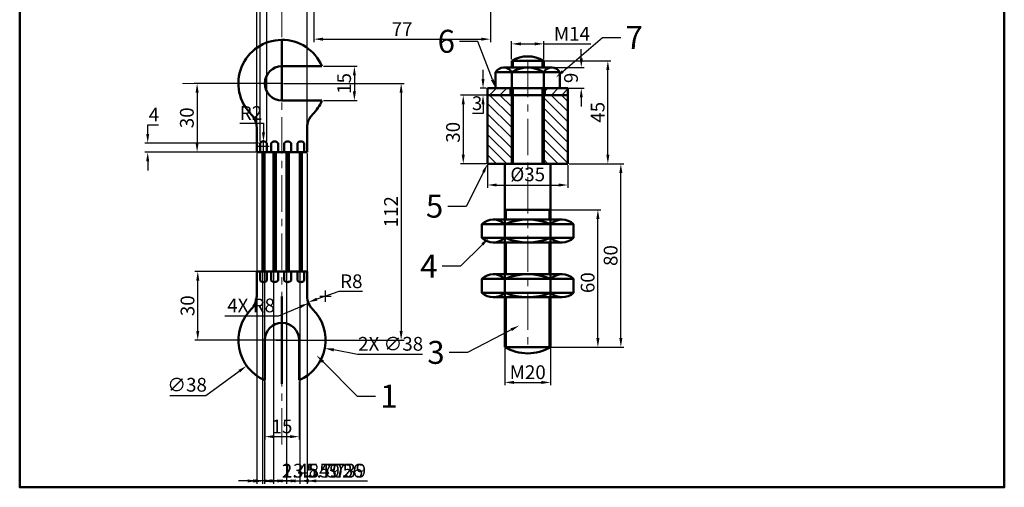
# Model space of a CAD drawing. Units: millimetres. Extents: x 297 to 727, y 87 to 537.
# Tile 1 of 2: x 297 to 727, y 87 to 291. Entities that reach past the tile are written whole.
import ezdxf
from ezdxf import colors
from ezdxf.entities.mleader import LeaderData, LeaderLine
from ezdxf.math import Vec2, Vec3

# ---------------------------------------------------------------- set-up
doc = ezdxf.new("R2010")
doc.units = ezdxf.units.MM
doc.header["$LTSCALE"] = 0.5
doc.linetypes.add('CENTER', pattern=[50.8, 31.75, -6.35, 6.35, -6.35])
for name, color, linetype, lineweight in [('M-CNTR', 1, 'CENTER', 18), ('M-DIMS', 2, 'Continuous', 25), ('M-HATC', 8, 'Continuous', 18), ('M-OUTL', 7, 'Continuous', 50), ('M-TEXT', 3, 'Continuous', 25), ('M-TTLB', 7, 'Continuous', 50)]:
    doc.layers.add(name, color=color, linetype=linetype, lineweight=lineweight)
doc.styles.get("Standard").update_dxf_attribs({"font": 'arial.ttf'})
doc.dimstyles.new('ISO-25', dxfattribs={"dimtxt": 6, "dimasz": 4, "dimexe": 1.25, "dimexo": 0.625, "dimtad": 1, "dimtoh": 1, "dimtxsty": 'Standard', "dimcen": 2.5, "dimadec": 0, "dimazin": 0, "dimtfac": 1, "dimtofl": 0, "dimtmove": 0, "dimatfit": 3, "dimfxl": 1, "dimarcsym": 0})

# ---------------------------------------------------------------- blocks, each defined once
blk = doc.blocks.new('*D1')
at = {"layer": 'Defpoints', "color": 0, "transparency": 16777216}
for p in [(525.99, 280.54), (511.99, 273.2), (525.99, 273.2)]:
    blk.add_point(p, dxfattribs=at)
at = {"layer": 'M-DIMS', "color": 0, "lineweight": -2, "transparency": 16777216}
for p, q in [((511.99, 273.83), (511.99, 281.79)), ((515.99, 280.54), (521.99, 280.54)), ((525.99, 273.83), (525.99, 281.79)), ((525.99, 280.54), (546.52, 280.54))]:
    blk.add_line(p, q, dxfattribs=at)
at = {"layer": 'M-DIMS', "color": 0, "transparency": 16777216}
for points in [[(515.99, 281.21), (515.99, 279.88), (511.99, 280.54)], [(521.99, 281.21), (521.99, 279.88), (525.99, 280.54)]]:
    blk.add_solid(points, dxfattribs=at)
at = {"layer": 'M-DIMS', "color": 0, "transparency": 16777216, "insert": (538.26, 284.18), "char_height": 6, "attachment_point": 5}
blk.add_mtext('M14', dxfattribs=at)
blk = doc.blocks.new('*D2')
at = {"layer": 'Defpoints', "color": 0, "transparency": 16777216}
for p in [(508.38, 270.2), (542.34, 270.2), (504.99, 261.2)]:
    blk.add_point(p, dxfattribs=at)
at = {"layer": 'M-DIMS', "color": 0, "lineweight": -2, "transparency": 16777216}
for p, q in [((542.34, 274.2), (542.34, 278.2)), ((509.01, 270.2), (543.59, 270.2)), ((505.62, 261.2), (543.59, 261.2)), ((542.34, 257.2), (542.34, 253.2))]:
    blk.add_line(p, q, dxfattribs=at)
at = {"layer": 'M-DIMS', "color": 0, "transparency": 16777216}
for points in [[(541.68, 274.2), (543.01, 274.2), (542.34, 270.2)], [(541.68, 257.2), (543.01, 257.2), (542.34, 261.2)]]:
    blk.add_solid(points, dxfattribs=at)
at = {"layer": 'M-DIMS', "color": 0, "transparency": 16777216, "insert": (538.66, 265.7), "char_height": 6, "attachment_point": 5, "rotation": 90}
blk.add_mtext('9', dxfattribs=at)
blk = doc.blocks.new('*D3')
at = {"layer": 'Defpoints', "color": 0, "transparency": 16777216}
for p in [(499.5, 258.2), (501.49, 261.2), (501.49, 258.2)]:
    blk.add_point(p, dxfattribs=at)
at = {"layer": 'M-DIMS', "color": 0, "lineweight": -2, "transparency": 16777216}
for p, q in [((499.5, 265.2), (499.5, 269.2)), ((500.87, 261.2), (498.25, 261.2)), ((500.87, 258.2), (498.25, 258.2)), ((499.5, 254.2), (499.5, 250.2)), ((499.5, 250.2), (494.95, 250.2))]:
    blk.add_line(p, q, dxfattribs=at)
at = {"layer": 'M-DIMS', "color": 0, "transparency": 16777216}
for points in [[(498.83, 265.2), (500.17, 265.2), (499.5, 261.2)], [(498.83, 254.2), (500.17, 254.2), (499.5, 258.2)]]:
    blk.add_solid(points, dxfattribs=at)
at = {"layer": 'M-DIMS', "color": 0, "transparency": 16777216, "insert": (496.91, 253.89), "char_height": 6, "attachment_point": 5}
blk.add_mtext('3', dxfattribs=at)
blk = doc.blocks.new('*D4')
at = {"layer": 'Defpoints', "color": 0, "transparency": 16777216}
for p in [(501.49, 258.2), (490.87, 228.2), (501.49, 228.2)]:
    blk.add_point(p, dxfattribs=at)
at = {"layer": 'M-DIMS', "color": 0, "lineweight": -2, "transparency": 16777216}
for p, q in [((500.87, 258.2), (489.62, 258.2)), ((490.87, 254.2), (490.87, 232.2)), ((500.87, 228.2), (489.62, 228.2))]:
    blk.add_line(p, q, dxfattribs=at)
at = {"layer": 'M-DIMS', "color": 0, "transparency": 16777216}
for points in [[(490.21, 254.2), (491.54, 254.2), (490.87, 258.2)], [(490.21, 232.2), (491.54, 232.2), (490.87, 228.2)]]:
    blk.add_solid(points, dxfattribs=at)
at = {"layer": 'M-DIMS', "color": 0, "transparency": 16777216, "insert": (487.18, 241.96), "char_height": 6, "attachment_point": 5, "rotation": 90}
blk.add_mtext('30', dxfattribs=at)
blk = doc.blocks.new('*D5')
at = {"layer": 'Defpoints', "color": 0, "transparency": 16777216}
for p in [(518.99, 273.2), (553.94, 273.2), (536.49, 228.2)]:
    blk.add_point(p, dxfattribs=at)
at = {"layer": 'M-DIMS', "color": 0, "lineweight": -2, "transparency": 16777216}
for p, q in [((519.62, 273.2), (555.19, 273.2)), ((553.94, 232.2), (553.94, 269.2)), ((537.12, 228.2), (555.19, 228.2))]:
    blk.add_line(p, q, dxfattribs=at)
at = {"layer": 'M-DIMS', "color": 0, "transparency": 16777216}
for points in [[(553.27, 269.2), (554.6, 269.2), (553.94, 273.2)], [(553.27, 232.2), (554.6, 232.2), (553.94, 228.2)]]:
    blk.add_solid(points, dxfattribs=at)
at = {"layer": 'M-DIMS', "color": 0, "transparency": 16777216, "insert": (550.26, 250.7), "char_height": 6, "attachment_point": 5, "rotation": 90}
blk.add_mtext('45', dxfattribs=at)
blk = doc.blocks.new('*D6')
at = {"layer": 'Defpoints', "color": 0, "transparency": 16777216}
for p in [(501.49, 228.2), (536.49, 228.2), (536.49, 218.97)]:
    blk.add_point(p, dxfattribs=at)
at = {"layer": 'M-DIMS', "color": 0, "lineweight": -2, "transparency": 16777216}
for p, q in [((501.49, 227.58), (501.49, 217.72)), ((536.49, 227.58), (536.49, 217.72)), ((505.49, 218.97), (532.49, 218.97))]:
    blk.add_line(p, q, dxfattribs=at)
at = {"layer": 'M-DIMS', "color": 0, "transparency": 16777216}
for points in [[(505.49, 219.63), (505.49, 218.3), (501.49, 218.97)], [(532.49, 219.63), (532.49, 218.3), (536.49, 218.97)]]:
    blk.add_solid(points, dxfattribs=at)
at = {"layer": 'M-DIMS', "color": 0, "transparency": 16777216, "insert": (518.99, 222.82), "char_height": 6, "attachment_point": 5}
blk.add_mtext('%%C35', dxfattribs=at)
blk = doc.blocks.new('*D7')
at = {"layer": 'Defpoints', "color": 0, "transparency": 16777216}
for p in [(518.99, 208.2), (549.59, 208.2), (518.99, 148.2)]:
    blk.add_point(p, dxfattribs=at)
at = {"layer": 'M-DIMS', "color": 0, "lineweight": -2, "transparency": 16777216}
for p, q in [((519.62, 208.2), (550.84, 208.2)), ((549.59, 152.2), (549.59, 204.2)), ((519.62, 148.2), (550.84, 148.2))]:
    blk.add_line(p, q, dxfattribs=at)
at = {"layer": 'M-DIMS', "color": 0, "transparency": 16777216}
for points in [[(548.92, 204.2), (550.26, 204.2), (549.59, 208.2)], [(548.92, 152.2), (550.26, 152.2), (549.59, 148.2)]]:
    blk.add_solid(points, dxfattribs=at)
at = {"layer": 'M-DIMS', "color": 0, "transparency": 16777216, "insert": (545.9, 176.36), "char_height": 6, "attachment_point": 5, "rotation": 90}
blk.add_mtext('60', dxfattribs=at)
blk = doc.blocks.new('*D8')
at = {"layer": 'Defpoints', "color": 0, "transparency": 16777216}
for p in [(536.49, 228.2), (559.61, 228.2), (518.99, 148.2)]:
    blk.add_point(p, dxfattribs=at)
at = {"layer": 'M-DIMS', "color": 0, "lineweight": -2, "transparency": 16777216}
for p, q in [((537.12, 228.2), (560.86, 228.2)), ((559.61, 152.2), (559.61, 224.2)), ((519.62, 148.2), (560.86, 148.2))]:
    blk.add_line(p, q, dxfattribs=at)
at = {"layer": 'M-DIMS', "color": 0, "transparency": 16777216}
for points in [[(558.94, 224.2), (560.28, 224.2), (559.61, 228.2)], [(558.94, 152.2), (560.28, 152.2), (559.61, 148.2)]]:
    blk.add_solid(points, dxfattribs=at)
at = {"layer": 'M-DIMS', "color": 0, "transparency": 16777216, "insert": (555.92, 188.2), "char_height": 6, "attachment_point": 5, "rotation": 90}
blk.add_mtext('80', dxfattribs=at)
blk = doc.blocks.new('*D9')
at = {"layer": 'Defpoints', "color": 0, "transparency": 16777216}
for p in [(508.99, 148.2), (528.99, 148.2), (528.99, 132.83)]:
    blk.add_point(p, dxfattribs=at)
at = {"layer": 'M-DIMS', "color": 0, "lineweight": -2, "transparency": 16777216}
for p, q in [((508.99, 147.58), (508.99, 131.58)), ((528.99, 147.58), (528.99, 131.58)), ((512.99, 132.83), (524.99, 132.83))]:
    blk.add_line(p, q, dxfattribs=at)
at = {"layer": 'M-DIMS', "color": 0, "transparency": 16777216}
for points in [[(512.99, 133.5), (512.99, 132.17), (508.99, 132.83)], [(524.99, 133.5), (524.99, 132.17), (528.99, 132.83)]]:
    blk.add_solid(points, dxfattribs=at)
at = {"layer": 'M-DIMS', "color": 0, "transparency": 16777216, "insert": (518.99, 136.52), "char_height": 6, "attachment_point": 5}
blk.add_mtext('M20', dxfattribs=at)
blk = doc.blocks.new('*D10')
at = {"layer": 'Defpoints', "color": 0, "transparency": 16777216}
for p in [(429.27, 270.79), (429.27, 255.79), (443.4, 255.79)]:
    blk.add_point(p, dxfattribs=at)
at = {"layer": 'M-DIMS', "color": 0, "lineweight": -2, "transparency": 16777216}
for p, q in [((429.9, 270.79), (444.65, 270.79)), ((443.4, 266.79), (443.4, 259.79)), ((429.9, 255.79), (444.65, 255.79))]:
    blk.add_line(p, q, dxfattribs=at)
at = {"layer": 'M-DIMS', "color": 0, "transparency": 16777216}
for points in [[(442.74, 266.79), (444.07, 266.79), (443.4, 270.79)], [(442.74, 259.79), (444.07, 259.79), (443.4, 255.79)]]:
    blk.add_solid(points, dxfattribs=at)
at = {"layer": 'M-DIMS', "color": 0, "transparency": 16777216, "insert": (439.71, 263.29), "char_height": 6, "attachment_point": 5, "rotation": 90}
blk.add_mtext('15', dxfattribs=at)
blk = doc.blocks.new('*D11')
at = {"layer": 'Defpoints', "color": 0, "transparency": 16777216}
for p in [(411.82, 263.29), (374.81, 233.29), (411.82, 233.29)]:
    blk.add_point(p, dxfattribs=at)
at = {"layer": 'M-DIMS', "color": 0, "lineweight": -2, "transparency": 16777216}
for p, q in [((411.19, 263.29), (373.56, 263.29)), ((374.81, 259.29), (374.81, 237.29)), ((411.19, 233.29), (373.56, 233.29))]:
    blk.add_line(p, q, dxfattribs=at)
at = {"layer": 'M-DIMS', "color": 0, "transparency": 16777216}
for points in [[(374.14, 259.29), (375.48, 259.29), (374.81, 263.29)], [(374.14, 237.29), (375.48, 237.29), (374.81, 233.29)]]:
    blk.add_solid(points, dxfattribs=at)
at = {"layer": 'M-DIMS', "color": 0, "transparency": 16777216, "insert": (371.12, 248.29), "char_height": 6, "attachment_point": 5, "rotation": 90}
blk.add_mtext('30', dxfattribs=at)
blk = doc.blocks.new('*D12')
at = {"layer": 'Defpoints', "color": 0, "transparency": 16777216}
for p in [(375.1, 181.29), (411.82, 181.29), (411.82, 151.29)]:
    blk.add_point(p, dxfattribs=at)
at = {"layer": 'M-DIMS', "color": 0, "lineweight": -2, "transparency": 16777216}
for p, q in [((411.19, 181.29), (373.85, 181.29)), ((375.1, 155.29), (375.1, 177.29)), ((411.19, 151.29), (373.85, 151.29))]:
    blk.add_line(p, q, dxfattribs=at)
at = {"layer": 'M-DIMS', "color": 0, "transparency": 16777216}
for points in [[(374.44, 177.29), (375.77, 177.29), (375.1, 181.29)], [(374.44, 155.29), (375.77, 155.29), (375.1, 151.29)]]:
    blk.add_solid(points, dxfattribs=at)
at = {"layer": 'M-DIMS', "color": 0, "transparency": 16777216, "insert": (371.41, 166.29), "char_height": 6, "attachment_point": 5, "rotation": 90}
blk.add_mtext('30', dxfattribs=at)
blk = doc.blocks.new('*D13')
at = {"layer": 'Defpoints', "color": 0, "transparency": 16777216}
for p in [(404.32, 133.83), (419.32, 133.83), (419.32, 109.19)]:
    blk.add_point(p, dxfattribs=at)
at = {"layer": 'M-DIMS', "color": 0, "lineweight": -2, "transparency": 16777216}
for p, q in [((404.32, 133.21), (404.32, 107.94)), ((419.32, 133.21), (419.32, 107.94)), ((408.32, 109.19), (415.32, 109.19))]:
    blk.add_line(p, q, dxfattribs=at)
at = {"layer": 'M-DIMS', "color": 0, "transparency": 16777216}
for points in [[(408.32, 109.85), (408.32, 108.52), (404.32, 109.19)], [(415.32, 109.85), (415.32, 108.52), (419.32, 109.19)]]:
    blk.add_solid(points, dxfattribs=at)
at = {"layer": 'M-DIMS', "color": 0, "transparency": 16777216, "insert": (411.82, 112.88), "char_height": 6, "attachment_point": 5}
blk.add_mtext('15', dxfattribs=at)
blk = doc.blocks.new('*D14')
at = {"layer": 'Defpoints', "color": 0, "transparency": 16777216}
for p in [(427.19, 162.46), (396.45, 140.12)]:
    blk.add_point(p, dxfattribs=at)
at = {"layer": 'M-DIMS', "color": 0, "lineweight": -2, "transparency": 16777216}
for p, q in [((409.32, 151.29), (414.32, 151.29)), ((411.82, 148.79), (411.82, 153.79)), ((378.65, 127.19), (393.21, 137.77)), ((362.89, 127.19), (378.65, 127.19))]:
    blk.add_line(p, q, dxfattribs=at)
at = {"layer": 'M-DIMS', "color": 0, "transparency": 16777216}
blk.add_solid([(392.82, 138.31), (393.6, 137.23), (396.45, 140.12)], dxfattribs=at)
at = {"layer": 'M-DIMS', "color": 0, "transparency": 16777216, "insert": (370.45, 131.04), "char_height": 6, "attachment_point": 5}
blk.add_mtext('∅38', dxfattribs=at)
blk = doc.blocks.new('*D15')
at = {"layer": 'Defpoints', "color": 0, "transparency": 16777216}
for p in [(423.27, 167.83), (430.82, 170.48)]:
    blk.add_point(p, dxfattribs=at)
at = {"layer": 'M-DIMS', "color": 0, "lineweight": -2, "transparency": 16777216}
for p, q in [((436.6, 172.5), (427.04, 169.15)), ((446.91, 172.5), (436.6, 172.5))]:
    blk.add_line(p, q, dxfattribs=at)
at = {"layer": 'M-DIMS', "color": 0, "transparency": 16777216}
blk.add_solid([(426.82, 169.78), (427.26, 168.52), (423.27, 167.83)], dxfattribs=at)
at = {"layer": 'M-DIMS', "color": 0, "transparency": 16777216, "insert": (442.07, 176.19), "char_height": 6, "attachment_point": 5}
blk.add_mtext('R8', dxfattribs=at)
blk = doc.blocks.new('*D16')
at = {"layer": 'Defpoints', "color": 0, "ltscale": 0.5, "transparency": 16777216}
for p in [(411.82, 263.29), (411.82, 151.29), (463.8, 151.29)]:
    blk.add_point(p, dxfattribs=at)
at = {"layer": 'M-DIMS', "color": 0, "lineweight": -2, "ltscale": 0.5, "transparency": 16777216}
for p, q in [((412.44, 263.29), (465.05, 263.29)), ((463.8, 259.29), (463.8, 155.29)), ((412.44, 151.29), (465.05, 151.29))]:
    blk.add_line(p, q, dxfattribs=at)
at = {"layer": 'M-DIMS', "color": 0, "ltscale": 0.5, "transparency": 16777216}
for points in [[(463.13, 259.29), (464.46, 259.29), (463.8, 263.29)], [(463.13, 155.29), (464.46, 155.29), (463.8, 151.29)]]:
    blk.add_solid(points, dxfattribs=at)
at = {"layer": 'M-DIMS', "color": 0, "ltscale": 0.5, "transparency": 16777216, "insert": (460.16, 207.29), "char_height": 6, "attachment_point": 5, "rotation": 90}
blk.add_mtext('112', dxfattribs=at)
blk = doc.blocks.new('NUT-HEX-M20')
for p, q in [((30, 2), (30, 10)), ((0, 2), (0, 8)), ((0, 8), (40, 8)), ((10, 2), (10, 8)), ((40, 8), (40, 2)), ((40, 2), (0, 2))]:
    blk.add_line(p, q)
for centre, radius, start, end in [((5, 2.75), 7.25, 46.3972, 133.6028), ((20, -16), 26, 67.3801, 112.6199), ((35, 2.75), 7.25, 46.3972, 133.6028), ((5, 7.25), 7.25, 226.3972, 313.6028), ((20, 26), 26, 247.3801, 292.6199), ((35, 7.25), 7.25, 226.3972, 313.6028)]:
    blk.add_arc(centre, radius, start, end)
blk = doc.blocks.new('WIRE-STRAND-END')
for p, q in [((0, 4.68), (0, 0.68)), ((3, 0.68), (3, 4.68))]:
    blk.add_line(p, q)
blk.add_arc((1.5, 2), 2, 221.4096, 318.5904)
blk = doc.blocks.new('BOLT-END-DOME')
for p, q in [((0, 3), (0, 0)), ((0, 3), (14, 3)), ((14, 3), (14, 0))]:
    blk.add_line(p, q)
blk.add_arc((7, -9.12), 14, 60, 120)
blk = doc.blocks.new('*D23')
at = {"layer": 'Defpoints', "color": 0, "ltscale": 0.5, "transparency": 16777216}
for p in [(425.71, 301.75), (502.71, 303.24), (502.71, 282.6)]:
    blk.add_point(p, dxfattribs=at)
at = {"layer": 'M-DIMS', "color": 0, "lineweight": -2, "ltscale": 0.5, "transparency": 16777216}
for p, q in [((425.71, 301.12), (425.71, 281.35)), ((502.71, 302.61), (502.71, 281.35)), ((429.71, 282.6), (498.71, 282.6))]:
    blk.add_line(p, q, dxfattribs=at)
at = {"layer": 'M-DIMS', "color": 0, "ltscale": 0.5, "transparency": 16777216}
for points in [[(429.71, 283.27), (429.71, 281.93), (425.71, 282.6)], [(498.71, 283.27), (498.71, 281.93), (502.71, 282.6)]]:
    blk.add_solid(points, dxfattribs=at)
at = {"layer": 'M-DIMS', "color": 0, "ltscale": 0.5, "transparency": 16777216, "insert": (464.21, 286.22), "char_height": 6, "attachment_point": 5}
blk.add_mtext('77', dxfattribs=at)
blk = doc.blocks.new('*D28')
at = {"layer": 'Defpoints', "color": 0, "ltscale": 0.5, "transparency": 16777216}
for p in [(422.82, 314.56), (400.82, 244.11), (422.82, 244.11)]:
    blk.add_point(p, dxfattribs=at)
at = {"layer": 'M-DIMS', "color": 0, "lineweight": -2, "ltscale": 0.5, "transparency": 16777216}
for p, q in [((400.82, 244.73), (400.82, 315.81)), ((404.82, 314.56), (418.82, 314.56)), ((422.82, 244.73), (422.82, 315.81))]:
    blk.add_line(p, q, dxfattribs=at)
at = {"layer": 'M-DIMS', "color": 0, "ltscale": 0.5, "transparency": 16777216}
for points in [[(404.82, 315.23), (404.82, 313.89), (400.82, 314.56)], [(418.82, 315.23), (418.82, 313.89), (422.82, 314.56)]]:
    blk.add_solid(points, dxfattribs=at)
at = {"layer": 'M-DIMS', "color": 0, "ltscale": 0.5, "transparency": 16777216, "insert": (411.82, 318.2), "char_height": 6, "attachment_point": 5}
blk.add_mtext('22', dxfattribs=at)
blk = doc.blocks.new('*D29')
at = {"layer": 'Defpoints', "color": 0, "ltscale": 0.5, "transparency": 16777216}
for p in [(400.82, 233.29), (403.26, 233.29), (403.26, 89.87)]:
    blk.add_point(p, dxfattribs=at)
at = {"layer": 'M-DIMS', "color": 0, "lineweight": -2, "ltscale": 0.5, "transparency": 16777216}
for p, q in [((400.82, 232.67), (400.82, 88.62)), ((403.26, 232.67), (403.26, 88.62)), ((396.82, 89.87), (392.82, 89.87)), ((407.26, 89.87), (428.24, 89.87))]:
    blk.add_line(p, q, dxfattribs=at)
at = {"layer": 'M-DIMS', "color": 0, "ltscale": 0.5, "transparency": 16777216}
for points in [[(396.82, 90.54), (396.82, 89.2), (400.82, 89.87)], [(407.26, 90.54), (407.26, 89.2), (403.26, 89.87)]]:
    blk.add_solid(points, dxfattribs=at)
at = {"layer": 'M-DIMS', "color": 0, "ltscale": 0.5, "transparency": 16777216, "insert": (419.75, 93.56), "char_height": 6, "attachment_point": 5}
blk.add_mtext('2.45', dxfattribs=at)
blk = doc.blocks.new('*D30')
at = {"layer": 'Defpoints', "color": 0, "ltscale": 0.5, "transparency": 16777216}
for p in [(403.26, 233.29), (404.26, 233.29), (404.26, 89.87)]:
    blk.add_point(p, dxfattribs=at)
at = {"layer": 'M-DIMS', "color": 0, "lineweight": -2, "ltscale": 0.5, "transparency": 16777216}
for p, q in [((403.26, 232.67), (403.26, 88.62)), ((404.26, 232.67), (404.26, 88.62)), ((399.26, 89.87), (395.26, 89.87)), ((408.26, 89.87), (415.72, 89.87))]:
    blk.add_line(p, q, dxfattribs=at)
at = {"layer": 'M-DIMS', "color": 0, "ltscale": 0.5, "transparency": 16777216}
for points in [[(399.26, 90.54), (399.26, 89.2), (403.26, 89.87)], [(408.26, 90.54), (408.26, 89.2), (404.26, 89.87)]]:
    blk.add_solid(points, dxfattribs=at)
at = {"layer": 'M-DIMS', "color": 0, "ltscale": 0.5, "transparency": 16777216, "insert": (413.99, 93.51), "char_height": 6, "attachment_point": 5}
blk.add_mtext('1', dxfattribs=at)
blk = doc.blocks.new('*D31')
at = {"layer": 'Defpoints', "color": 0, "ltscale": 0.5, "transparency": 16777216}
for p in [(404.26, 233.29), (408.11, 233.29), (408.11, 89.87)]:
    blk.add_point(p, dxfattribs=at)
at = {"layer": 'M-DIMS', "color": 0, "lineweight": -2, "ltscale": 0.5, "transparency": 16777216}
for p, q in [((404.26, 232.67), (404.26, 88.62)), ((408.11, 232.67), (408.11, 88.62)), ((400.26, 89.87), (396.26, 89.87)), ((412.11, 89.87), (437.62, 89.87))]:
    blk.add_line(p, q, dxfattribs=at)
at = {"layer": 'M-DIMS', "color": 0, "ltscale": 0.5, "transparency": 16777216}
for points in [[(400.26, 90.54), (400.26, 89.2), (404.26, 89.87)], [(412.11, 90.54), (412.11, 89.2), (408.11, 89.87)]]:
    blk.add_solid(points, dxfattribs=at)
at = {"layer": 'M-DIMS', "color": 0, "ltscale": 0.5, "transparency": 16777216, "insert": (426.86, 93.56), "char_height": 6, "attachment_point": 5}
blk.add_mtext('3.849', dxfattribs=at)
blk = doc.blocks.new('*D32')
at = {"layer": 'Defpoints', "color": 0, "ltscale": 0.5, "transparency": 16777216}
for p in [(408.11, 233.29), (413.82, 233.29), (413.82, 89.87)]:
    blk.add_point(p, dxfattribs=at)
at = {"layer": 'M-DIMS', "color": 0, "lineweight": -2, "ltscale": 0.5, "transparency": 16777216}
for p, q in [((408.11, 232.67), (408.11, 88.62)), ((413.82, 232.67), (413.82, 88.62)), ((404.11, 89.87), (400.11, 89.87)), ((417.82, 89.87), (443.36, 89.87))]:
    blk.add_line(p, q, dxfattribs=at)
at = {"layer": 'M-DIMS', "color": 0, "ltscale": 0.5, "transparency": 16777216}
for points in [[(404.11, 90.54), (404.11, 89.2), (408.11, 89.87)], [(417.82, 90.54), (417.82, 89.2), (413.82, 89.87)]]:
    blk.add_solid(points, dxfattribs=at)
at = {"layer": 'M-DIMS', "color": 0, "ltscale": 0.5, "transparency": 16777216, "insert": (432.59, 93.56), "char_height": 6, "attachment_point": 5}
blk.add_mtext('5.705', dxfattribs=at)
blk = doc.blocks.new('*D33')
at = {"layer": 'Defpoints', "color": 0, "ltscale": 0.5, "transparency": 16777216}
for p in [(413.82, 233.29), (419.55, 233.29), (419.55, 89.87)]:
    blk.add_point(p, dxfattribs=at)
at = {"layer": 'M-DIMS', "color": 0, "lineweight": -2, "ltscale": 0.5, "transparency": 16777216}
for p, q in [((413.82, 232.67), (413.82, 88.62)), ((419.55, 232.67), (419.55, 88.62)), ((409.82, 89.87), (405.82, 89.87)), ((423.55, 89.87), (449.06, 89.87))]:
    blk.add_line(p, q, dxfattribs=at)
at = {"layer": 'M-DIMS', "color": 0, "ltscale": 0.5, "transparency": 16777216}
for points in [[(409.82, 90.54), (409.82, 89.2), (413.82, 89.87)], [(423.55, 90.54), (423.55, 89.2), (419.55, 89.87)]]:
    blk.add_solid(points, dxfattribs=at)
at = {"layer": 'M-DIMS', "color": 0, "ltscale": 0.5, "transparency": 16777216, "insert": (438.31, 93.56), "char_height": 6, "attachment_point": 5}
blk.add_mtext('5.739', dxfattribs=at)
blk = doc.blocks.new('*D34')
at = {"layer": 'Defpoints', "color": 0, "ltscale": 0.5, "transparency": 16777216}
for p in [(419.55, 233.29), (422.82, 233.29), (422.82, 89.87)]:
    blk.add_point(p, dxfattribs=at)
at = {"layer": 'M-DIMS', "color": 0, "lineweight": -2, "ltscale": 0.5, "transparency": 16777216}
for p, q in [((419.55, 232.67), (419.55, 88.62)), ((422.82, 232.67), (422.82, 88.62)), ((415.55, 89.87), (411.55, 89.87)), ((426.82, 89.87), (447.64, 89.87))]:
    blk.add_line(p, q, dxfattribs=at)
at = {"layer": 'M-DIMS', "color": 0, "ltscale": 0.5, "transparency": 16777216}
for points in [[(415.55, 90.54), (415.55, 89.2), (419.55, 89.87)], [(426.82, 90.54), (426.82, 89.2), (422.82, 89.87)]]:
    blk.add_solid(points, dxfattribs=at)
at = {"layer": 'M-DIMS', "color": 0, "ltscale": 0.5, "transparency": 16777216, "insert": (439.23, 93.56), "char_height": 6, "attachment_point": 5}
blk.add_mtext('3.26', dxfattribs=at)
blk = doc.blocks.new('*D35')
at = {"layer": 'Defpoints', "color": 0, "ltscale": 0.5, "transparency": 16777216}
for p in [(405.26, 314.56), (402.26, 237.29), (405.26, 237.29)]:
    blk.add_point(p, dxfattribs=at)
at = {"layer": 'M-DIMS', "color": 0, "lineweight": -2, "ltscale": 0.5, "transparency": 16777216}
for p, q in [((398.26, 314.56), (394.26, 314.56)), ((402.26, 237.92), (402.26, 315.81)), ((405.26, 237.92), (405.26, 315.81)), ((409.26, 314.56), (418.44, 314.56))]:
    blk.add_line(p, q, dxfattribs=at)
at = {"layer": 'M-DIMS', "color": 0, "ltscale": 0.5, "transparency": 16777216}
for points in [[(398.26, 315.23), (398.26, 313.89), (402.26, 314.56)], [(409.26, 315.23), (409.26, 313.89), (405.26, 314.56)]]:
    blk.add_solid(points, dxfattribs=at)
at = {"layer": 'M-DIMS', "color": 0, "ltscale": 0.5, "transparency": 16777216, "insert": (415.85, 318.25), "char_height": 6, "attachment_point": 5}
blk.add_mtext('3', dxfattribs=at)
blk = doc.blocks.new('*D36')
at = {"layer": 'Defpoints', "color": 0, "ltscale": 0.5, "transparency": 16777216}
for p in [(353.28, 237.29), (402.26, 237.29), (402.26, 233.29)]:
    blk.add_point(p, dxfattribs=at)
at = {"layer": 'M-DIMS', "color": 0, "lineweight": -2, "ltscale": 0.5, "transparency": 16777216}
for p, q in [((353.28, 241.29), (353.28, 245.29)), ((353.28, 245.29), (358.05, 245.29)), ((401.64, 237.29), (352.03, 237.29)), ((401.64, 233.29), (352.03, 233.29)), ((353.28, 229.29), (353.28, 225.29))]:
    blk.add_line(p, q, dxfattribs=at)
at = {"layer": 'M-DIMS', "color": 0, "ltscale": 0.5, "transparency": 16777216}
for points in [[(352.61, 241.29), (353.94, 241.29), (353.28, 237.29)], [(352.61, 229.29), (353.94, 229.29), (353.28, 233.29)]]:
    blk.add_solid(points, dxfattribs=at)
at = {"layer": 'M-DIMS', "color": 0, "ltscale": 0.5, "transparency": 16777216, "insert": (355.98, 248.92), "char_height": 6, "attachment_point": 5}
blk.add_mtext('4', dxfattribs=at)
blk = doc.blocks.new('*D43')
at = {"layer": 'Defpoints', "color": 0, "ltscale": 0.5, "transparency": 16777216}
for p in [(393.15, 154.83), (430.48, 147.75)]:
    blk.add_point(p, dxfattribs=at)
at = {"layer": 'M-DIMS', "color": 0, "lineweight": -2, "ltscale": 0.5, "transparency": 16777216}
for p, q in [((409.32, 151.29), (414.32, 151.29)), ((411.82, 148.79), (411.82, 153.79)), ((444.69, 145.06), (434.41, 147.01)), ((473.13, 145.06), (444.69, 145.06))]:
    blk.add_line(p, q, dxfattribs=at)
at = {"layer": 'M-DIMS', "color": 0, "ltscale": 0.5, "transparency": 16777216}
blk.add_solid([(434.54, 147.66), (434.29, 146.35), (430.48, 147.75)], dxfattribs=at)
at = {"layer": 'M-DIMS', "color": 0, "ltscale": 0.5, "transparency": 16777216, "insert": (459.22, 148.91), "char_height": 6, "attachment_point": 5}
blk.add_mtext('2X ∅38', dxfattribs=at)
blk = doc.blocks.new('*D44')
at = {"layer": 'Defpoints', "color": 0, "ltscale": 0.5, "transparency": 16777216}
for p in [(430.82, 170.48), (423.43, 167.4)]:
    blk.add_point(p, dxfattribs=at)
at = {"layer": 'M-DIMS', "color": 0, "lineweight": -2, "ltscale": 0.5, "transparency": 16777216}
for p, q in [((430.82, 167.98), (430.82, 172.98)), ((428.32, 170.48), (433.32, 170.48)), ((410.39, 161.96), (419.74, 165.86)), ((386.95, 161.96), (410.39, 161.96))]:
    blk.add_line(p, q, dxfattribs=at)
at = {"layer": 'M-DIMS', "color": 0, "ltscale": 0.5, "transparency": 16777216}
blk.add_solid([(419.48, 166.47), (420, 165.24), (423.43, 167.4)], dxfattribs=at)
at = {"layer": 'M-DIMS', "color": 0, "ltscale": 0.5, "transparency": 16777216, "insert": (398.36, 165.65), "char_height": 6, "attachment_point": 5}
blk.add_mtext('4X R8', dxfattribs=at)
blk = doc.blocks.new('*D45')
at = {"layer": 'Defpoints', "color": 0, "ltscale": 0.5, "transparency": 16777216}
for p in [(403.76, 237.97), (403.76, 235.97)]:
    blk.add_point(p, dxfattribs=at)
at = {"layer": 'M-DIMS', "color": 0, "lineweight": -2, "ltscale": 0.5, "transparency": 16777216}
for p, q in [((393.51, 245.97), (403.75, 245.97)), ((403.75, 245.97), (403.76, 241.97)), ((403.76, 233.47), (403.76, 238.47)), ((401.26, 235.97), (406.26, 235.97))]:
    blk.add_line(p, q, dxfattribs=at)
at = {"layer": 'M-DIMS', "color": 0, "ltscale": 0.5, "transparency": 16777216}
blk.add_solid([(404.42, 241.97), (403.09, 241.97), (403.76, 237.97)], dxfattribs=at)
at = {"layer": 'M-DIMS', "color": 0, "ltscale": 0.5, "transparency": 16777216, "insert": (398.32, 249.61), "char_height": 6, "attachment_point": 5}
blk.add_mtext('R2', dxfattribs=at)

msp = doc.modelspace()

# ---------------------------------------------------------------- hatches: boundary and pattern name
at = {"layer": 'M-HATC'}
h = msp.add_hatch(dxfattribs=at)
h.set_pattern_fill('ANSI31', color=256)
h.set_pattern_definition([(45, (-61.1634, 22.4378), (-2.245064, 2.245064), [])])
h.paths.add_polyline_path([(536.4914, 258.204), (536.4914, 261.204), (526.4914, 261.204), (526.4914, 258.204)])
h.paths.add_polyline_path([(511.4914, 258.204), (511.4914, 261.204), (501.4914, 261.204), (501.4914, 258.204)])
h = msp.add_hatch(dxfattribs=at)
h.set_pattern_fill('ANSI31', color=256, angle=90)
h.set_pattern_definition([(135, (-61.1634, 22.4378), (-2.245064, -2.245064), [])])
h.paths.add_polyline_path([(511.9914, 258.204), (501.4914, 258.204), (501.4914, 228.204), (511.9914, 228.204)])
h.paths.add_polyline_path([(536.4914, 258.204), (525.9914, 258.204), (525.9914, 228.204), (536.4914, 228.204)])

# ---------------------------------------------------------------- linework, layer by layer
at = {"layer": 'M-CNTR'}
for p, q in [((411.8162, 299.409), (411.8162, 105.0214)), ((518.9914, 273.204), (518.9914, 148.204)), ((368.425, 263.2918), (455.2074, 263.2918)), ((378.8584, 151.2918), (444.7739, 151.2918))]:
    msp.add_line(p, q, dxfattribs=at)
at = {"layer": 'M-OUTL'}
for p, q in [((411.8162, 282.2918), (411.8162, 255.7918)), ((411.8162, 270.7918), (429.2733, 270.7918)), ((512.4914, 273.204), (512.4914, 270.204)), ((525.4914, 273.204), (525.4914, 270.204)), ((504.9914, 261.204), (504.9914, 268.204)), ((504.9914, 268.204), (532.9914, 268.204)), ((508.3803, 270.204), (529.6025, 270.204)), ((511.9914, 268.204), (511.9914, 228.204)), ((525.9914, 268.204), (525.9914, 228.204)), ((532.9914, 261.204), (532.9914, 268.204)), ((501.4914, 261.204), (536.4914, 261.204)), ((501.4914, 228.204), (501.4914, 261.204)), ((501.4914, 258.204), (536.4914, 258.204)), ((511.4914, 258.204), (511.4914, 261.204)), ((512.4914, 261.204), (512.4914, 228.204)), ((525.4914, 261.204), (525.4914, 228.204)), ((526.4914, 258.204), (526.4914, 261.204)), ((536.4914, 261.204), (536.4914, 228.204)), ((411.8162, 255.7918), (429.2733, 255.7918)), ((400.8162, 244.1085), (400.8162, 233.2918)), ((422.8162, 233.2918), (422.8162, 244.1085)), ((400.8162, 233.2918), (422.8162, 233.2918)), ((403.2617, 233.2918), (403.2617, 181.2918)), ((404.2617, 233.2918), (404.2617, 181.2918)), ((408.1109, 233.2918), (408.1109, 181.2918)), ((409.1109, 233.2918), (409.1109, 181.2918)), ((413.8162, 233.2918), (413.8162, 181.2918)), ((414.8162, 233.2918), (414.8162, 181.2918)), ((419.5548, 233.2918), (419.5548, 181.2918)), ((420.5548, 233.2918), (420.5548, 181.2918)), ((536.4914, 228.204), (501.4914, 228.204)), ((508.9914, 228.204), (508.9914, 148.204)), ((528.9914, 228.204), (528.9914, 148.204)), ((528.9914, 208.204), (508.9914, 208.204)), ((509.4914, 208.204), (509.4914, 203.9075)), ((528.4914, 203.9075), (528.4914, 208.204)), ((503.9914, 203.9075), (533.9914, 203.9075)), ((533.9914, 193.9075), (503.9914, 193.9075)), ((509.4914, 179.9996), (509.4914, 193.9075)), ((528.4914, 193.9075), (528.4914, 179.9996)), ((400.8162, 181.2918), (422.8162, 181.2918)), ((400.8162, 181.2918), (400.8162, 170.4752)), ((422.8162, 181.2918), (422.8162, 170.4752)), ((503.9914, 179.9996), (533.9914, 179.9996)), ((411.8162, 170.2918), (411.8162, 132.2918)), ((533.9914, 169.9996), (503.9914, 169.9996)), ((509.4914, 169.9996), (509.4914, 148.204)), ((528.4914, 169.9996), (528.4914, 148.204)), ((404.3162, 151.2918), (404.3162, 133.8347)), ((419.3162, 151.2918), (419.3162, 133.8347)), ((528.9914, 148.204), (508.9914, 148.204))]:
    msp.add_line(p, q, dxfattribs=at)
for centre, radius, start, end in [((411.8162, 263.2918), 19, 23.249563, 225.275087), ((411.8162, 263.2918), 7.5, 90, 270), ((508.4914, 266.1446), 4.0609, 30.472735, 149.527265), ((518.9914, 256.954), 13.25, 58.109208, 121.890792), ((529.4914, 266.1446), 4.0609, 30.472735, 149.527265), ((411.8162, 263.2918), 19, 314.724913, 336.750437), ((392.8162, 244.1085), 8, 0, 45.275087), ((430.8162, 244.1085), 8, 134.724913, 180), ((392.8162, 170.4752), 8, 314.724913, 0), ((430.8162, 170.4752), 8, 180, 225.275087), ((411.8162, 151.2918), 19, 134.724913, 246.750437), ((411.8162, 151.2918), 19, 293.249563, 45.275087), ((411.8162, 151.2918), 7.5, 0, 180), ((518.9914, 165.5245), 20, 240, 300)]:
    msp.add_arc(centre, radius, start, end, dxfattribs=at)
at = {"layer": 'M-TTLB', "ltscale": 0.5}
msp.add_lwpolyline([(297.4476, 537.4188), (726.8242, 537.4188), (726.8242, 87.0773), (297.4476, 87.0773)], close=True, dxfattribs=at)

# ---------------------------------------------------------------- block references
at = {"layer": 'M-OUTL'}
for name, p in [('BOLT-END-DOME', (511.991, 270.204)), ('NUT-HEX-M20', (498.991, 193.907)), ('WIRE-STRAND-END', (402.2616, 176.615)), ('WIRE-STRAND-END', (407.1107, 176.615)), ('WIRE-STRAND-END', (412.816, 176.615)), ('WIRE-STRAND-END', (418.5546, 176.615)), ('NUT-HEX-M20', (498.991, 169.9991))]:
    msp.add_blockref(name, p, dxfattribs=at)
at = {"layer": 'M-OUTL', "rotation": 180}
for p in [(405.2619, 237.9687), (410.1111, 237.9687), (415.8164, 237.9687), (421.555, 237.9687)]:
    msp.add_blockref('WIRE-STRAND-END', p, dxfattribs=at)

# ---------------------------------------------------------------- dimensions: what is measured, and where the dimension line sits
at = {"layer": 'M-DIMS', "ltscale": 0.5}
for base, p1, p2, override, picture, middle in [((405.2617, 314.559), (402.2617, 237.2918), (405.2617, 237.2918), {"dimdec": 0, "dimlfac": 1, "dimrnd": 0, "dimzin": 0, "dimdsep": 46, "dimlunit": 2}, '*D35', (415.8513, 318.2495)), ((422.8162, 314.559), (400.8162, 244.1085), (422.8162, 244.1085), {"dimdec": 0, "dimlfac": 1, "dimrnd": 0, "dimzin": 0, "dimdsep": 46, "dimlunit": 2}, '*D28', (411.8162, 318.1963)), ((502.7052, 282.5987), (425.7052, 301.7487), (502.7052, 303.2378), {"dimdec": 0, "dimlfac": 1, "dimrnd": 0, "dimzin": 0, "dimdsep": 46, "dimlunit": 2}, '*D23', (464.2052, 286.2237)), ((403.2617, 89.8714), (400.8162, 233.2918), (403.2617, 233.2918), {"dimdec": 2, "dimlfac": 1, "dimrnd": 0, "dimzin": 0, "dimdsep": 46, "dimlunit": 2}, '*D29', (419.753, 93.5599)), ((404.2617, 89.8714), (403.2617, 233.2918), (404.2617, 233.2918), {"dimdec": 0, "dimlfac": 1, "dimrnd": 0, "dimzin": 0, "dimdsep": 46, "dimlunit": 2}, '*D30', (413.9918, 93.5087)), ((408.1109, 89.8714), (404.2617, 233.2918), (408.1109, 233.2918), {"dimdec": 3, "dimlfac": 1, "dimrnd": 0, "dimzin": 0, "dimdsep": 46, "dimlunit": 2}, '*D31', (426.8634, 93.5619)), ((413.8162, 89.8714), (408.1109, 233.2918), (413.8162, 233.2918), {"dimdec": 3, "dimlfac": 1, "dimrnd": 0, "dimzin": 0, "dimdsep": 46, "dimlunit": 2}, '*D32', (432.5872, 93.5599)), ((419.5548, 89.8714), (413.8162, 233.2918), (419.5548, 233.2918), {"dimdec": 3, "dimlfac": 1, "dimrnd": 0, "dimzin": 0, "dimdsep": 46, "dimlunit": 2}, '*D33', (438.3094, 93.5619)), ((422.8162, 89.8714), (419.5548, 233.2918), (422.8162, 233.2918), {"dimdec": 2, "dimlfac": 1, "dimrnd": 0, "dimzin": 0, "dimdsep": 46, "dimlunit": 2}, '*D34', (439.2297, 93.5619))]:
    dim = msp.add_linear_dim(base=base, p1=p1, p2=p2, dimstyle='ISO-25', override=override, dxfattribs=at)
    dim.commit()
    dim.dimension.update_dxf_attribs({"geometry": picture, "text_midpoint": middle})
at = {"layer": 'M-DIMS'}
for base, p1, p2, text, picture, middle in [((525.9914, 280.5442), (511.9914, 273.204), (525.9914, 273.204), 'M<>', '*D1', (538.2555, 284.1815)), ((536.4914, 218.9653), (501.4914, 228.204), (536.4914, 228.204), '%%C<>', '*D6', (518.9914, 222.8215)), ((528.9914, 132.8338), (508.9914, 148.204), (528.9914, 148.204), 'M<>', '*D9', (518.9914, 136.5222))]:
    dim = msp.add_linear_dim(base=base, p1=p1, p2=p2, text=text, dimstyle='ISO-25', override={"dimclrd": 0, "dimclre": 0, "dimclrt": 0}, dxfattribs=at)
    dim.commit()
    dim.dimension.update_dxf_attribs({"geometry": picture, "text_midpoint": middle})
for base, p1, p2, picture, middle in [((542.3436, 270.204), (504.9914, 261.204), (508.3803, 270.204), '*D2', (538.6552, 265.704)), ((443.4034, 255.7918), (429.2733, 270.7918), (429.2733, 255.7918), '*D10', (439.715, 263.2918)), ((553.9382, 273.204), (536.4914, 228.204), (518.9914, 273.204), '*D5', (550.262, 250.704)), ((499.5003, 258.204), (501.4914, 261.204), (501.4914, 258.204), '*D3', (496.9108, 253.8944)), ((374.8102, 233.2918), (411.8162, 263.2918), (411.8162, 233.2918), '*D11', (371.1198, 248.2918)), ((375.1026, 181.2918), (411.8162, 151.2918), (411.8162, 181.2918), '*D12', (371.4121, 166.2918))]:
    dim = msp.add_linear_dim(base=base, p1=p1, p2=p2, angle=90, dimstyle='ISO-25', override={"dimclrd": 0, "dimclre": 0, "dimclrt": 0}, dxfattribs=at)
    dim.commit()
    dim.dimension.update_dxf_attribs({"geometry": picture, "text_midpoint": middle})
at = {"layer": 'M-DIMS', "ltscale": 0.5}
for base, p1, p2, override, picture, middle in [((463.7953, 151.2918), (411.8162, 263.2918), (411.8162, 151.2918), {"dimclrd": 0, "dimclre": 0, "dimclrt": 0}, '*D16', (460.158, 207.2918)), ((353.275, 237.2918), (402.2617, 233.2918), (402.2617, 237.2918), {"dimdec": 0, "dimlfac": 1, "dimrnd": 0, "dimzin": 0, "dimdsep": 46, "dimlunit": 2}, '*D36', (355.975, 248.9168))]:
    dim = msp.add_linear_dim(base=base, p1=p1, p2=p2, angle=90, dimstyle='ISO-25', override=override, dxfattribs=at)
    dim.commit()
    dim.dimension.update_dxf_attribs({"geometry": picture, "text_midpoint": middle})
at = {"layer": 'M-DIMS'}
for base, p1, p2, picture, middle in [((490.8747, 228.204), (501.4914, 258.204), (501.4914, 228.204), '*D4', (490.8747, 241.9644)), ((559.6099, 228.204), (518.9914, 148.204), (536.4914, 228.204), '*D8', (559.6099, 188.204)), ((549.5889, 208.204), (518.9914, 148.204), (518.9914, 208.204), '*D7', (549.5889, 176.3554))]:
    dim = msp.add_linear_dim(base=base, p1=p1, p2=p2, angle=90, dimstyle='ISO-25', override={"dimclrd": 0, "dimclre": 0, "dimclrt": 0}, dxfattribs=at)
    dim.commit()
    dim.dimension.update_dxf_attribs({"geometry": picture, "text_midpoint": middle, "dimtype": 160})
at = {"layer": 'M-DIMS', "ltscale": 0.5}
dim = msp.add_radius_dim(center=(403.7617, 235.969), mpoint=(403.76, 237.969), dimstyle='ISO-25', override={"dimdec": 0, "dimlfac": 1, "dimrnd": 0, "dimzin": 0, "dimdsep": 46, "dimlunit": 2}, dxfattribs=at)
dim.commit()
dim.dimension.update_dxf_attribs({"geometry": '*D45', "text_midpoint": (398.3211, 249.6062)})
at = {"layer": 'M-DIMS'}
dim = msp.add_radius_dim(center=(430.8162, 170.4752), mpoint=(423.2676, 167.8257), dimstyle='ISO-25', override={"dimclrd": 0, "dimclre": 0, "dimclrt": 0}, dxfattribs=at)
dim.commit()
dim.dimension.update_dxf_attribs({"geometry": '*D15', "text_midpoint": (442.0661, 172.5043), "dimtype": 164})
at = {"layer": 'M-DIMS', "ltscale": 0.5}
dim = msp.add_radius_dim(center=(430.8162, 170.4752), mpoint=(423.4326, 167.3958), text='4X <>', dimstyle='ISO-25', override={"dimdec": 0, "dimlfac": 1, "dimrnd": 0, "dimzin": 0, "dimdsep": 46, "dimlunit": 2}, dxfattribs=at)
dim.commit()
dim.dimension.update_dxf_attribs({"geometry": '*D44', "text_midpoint": (398.3585, 165.6466)})
at = {"layer": 'M-DIMS'}
dim = msp.add_diameter_dim_2p(p1=(427.186, 162.4618), p2=(396.4464, 140.1218), dimstyle='ISO-25', override={"dimclrd": 0, "dimclre": 0, "dimclrt": 0}, dxfattribs=at)
dim.commit()
dim.dimension.update_dxf_attribs({"geometry": '*D14', "text_midpoint": (370.4542, 127.186), "dimtype": 163})
at = {"layer": 'M-DIMS', "ltscale": 0.5}
dim = msp.add_diameter_dim_2p(p1=(393.1488, 154.8316), p2=(430.4835, 147.7521), text='2X <>', dimstyle='ISO-25', override={"dimdec": 0, "dimlfac": 1, "dimrnd": 0, "dimzin": 0, "dimdsep": 46, "dimlunit": 2}, dxfattribs=at)
dim.commit()
dim.dimension.update_dxf_attribs({"geometry": '*D43', "text_midpoint": (444.6928, 145.0577), "dimtype": 163})
at = {"layer": 'M-DIMS'}
dim = msp.add_linear_dim(base=(419.3162, 109.1881), p1=(404.3162, 133.8347), p2=(419.3162, 133.8347), dimstyle='ISO-25', override={"dimclrd": 0, "dimclre": 0, "dimclrt": 0}, dxfattribs=at)
dim.commit()
dim.dimension.update_dxf_attribs({"geometry": '*D13', "text_midpoint": (411.8162, 112.8765)})

# ---------------------------------------------------------------- leaders
at = {"layer": 'M-TEXT', "ltscale": 0.5}
ml = msp.add_multileader_mtext('Standard', dxfattribs=at)
ml.set_content('CLAMPING NUT FOR \\PSLATE PLATE', color=256)
ml.set_leader_properties()
ml.build(insert=Vec2(0, 0))
ctx = ml.context
ctx.base_point, ctx.char_height, ctx.plane_origin = Vec3(551.7646, 355.6198), 10, Vec3(522.7052, 365.8764)
notes = []
notes.append((ctx, [(0, (1, 1, 0), (543.7646, 355.6198), (1, 0), 8, [(0, [(522.7052, 365.8764)], 0, [])])]))
ctx.mtext.insert, ctx.mtext.flow_direction = Vec3(553.7646, 360.7051), 5
ml = msp.add_multileader_mtext('Standard', dxfattribs=at)
ml.set_content('7', color=256)
ml.set_leader_properties()
ml.build(insert=Vec2(0, 0))
ctx = ml.context
ctx.base_point, ctx.char_height, ctx.plane_origin = Vec3(559.6609, 283.3714), 10, Vec3(531.2792, 265.9161)
notes.append((ctx, [(0, (1, 1, 0), (551.6609, 283.3714), (1, 0), 8, [(0, [(531.2792, 265.9161)], 0, [])])]))
ctx.mtext.insert, ctx.mtext.flow_direction = Vec3(561.6609, 288.3714), 5
ml = msp.add_multileader_mtext('Standard', dxfattribs=at)
ml.set_content('6', color=256)
ml.set_leader_properties()
ml.build(insert=Vec2(0, 0))
ctx = ml.context
ctx.base_point, ctx.char_height, ctx.plane_origin = Vec3(478.6636, 281.5876), 10, Vec3(504.9914, 261.204)
ctx.text_align_type = 2
notes.append((ctx, [(0, (1, 1, 0), (497.2666, 281.5876), (-1, 0), 8, [(0, [(504.9914, 261.204)], 0, [])])]))
ctx.mtext.insert, ctx.mtext.alignment, ctx.mtext.flow_direction = Vec3(487.2666, 286.6729), 3, 5
ml = msp.add_multileader_mtext('Standard', dxfattribs=at)
ml.set_content('5', color=256)
ml.set_leader_properties()
ml.build(insert=Vec2(0, 0))
ctx = ml.context
ctx.base_point, ctx.char_height, ctx.plane_origin = Vec3(473.5318, 209.6515), 10, Vec3(501.4914, 228.204)
ctx.text_align_type = 2
notes.append((ctx, [(0, (1, 1, 0), (492.1621, 209.6515), (-1, 0), 8, [(0, [(501.4914, 228.204)], 0, [])])]))
ctx.mtext.insert, ctx.mtext.alignment, ctx.mtext.flow_direction = Vec3(482.1621, 214.7368), 3, 5
ml = msp.add_multileader_mtext('Standard', dxfattribs=at)
ml.set_content('4', color=256)
ml.set_leader_properties()
ml.build(insert=Vec2(0, 0))
ctx = ml.context
ctx.base_point, ctx.char_height, ctx.plane_origin = Vec3(470.7523, 183.5264), 10, Vec3(502.0501, 195.9075)
ctx.text_align_type = 2
notes.append((ctx, [(0, (1, 1, 0), (489.6691, 183.5264), (-1, 0), 8, [(0, [(502.0501, 195.9075)], 0, [])])]))
ctx.mtext.insert, ctx.mtext.alignment, ctx.mtext.flow_direction = Vec3(479.6691, 188.5264), 3, 5
ml = msp.add_multileader_mtext('Standard', dxfattribs=at)
ml.set_content('3', color=256)
ml.set_leader_properties()
ml.build(insert=Vec2(0, 0))
ctx = ml.context
ctx.base_point, ctx.char_height, ctx.plane_origin = Vec3(474.207, 145.8548), 10, Vec3(515.3661, 157.7016)
ctx.text_align_type = 2
notes.append((ctx, [(0, (1, 1, 0), (492.7554, 145.8548), (-1, 0), 8, [(0, [(515.3661, 157.7016)], 0, [])])]))
ctx.mtext.insert, ctx.mtext.alignment, ctx.mtext.flow_direction = Vec3(482.7554, 150.9435), 3, 5
ml = msp.add_multileader_mtext('Standard', dxfattribs=at)
ml.set_content('1', color=256)
ml.set_leader_properties()
ml.build(insert=Vec2(0, 0))
ctx = ml.context
ctx.base_point, ctx.char_height, ctx.plane_origin = Vec3(452.6665, 126.88), 10, Vec3(426.8879, 144.6586)
notes.append((ctx, [(0, (1, 1, 0), (444.6665, 126.88), (1, 0), 8, [(0, [(426.8879, 144.6586)], 0, [])])]))
ctx.mtext.insert, ctx.mtext.flow_direction = Vec3(454.6665, 131.88), 5
for ctx, leaders in notes:
    for number, flags, end, landing, length, lines in leaders:
        leader = LeaderData()
        leader.index, (leader.has_last_leader_line, leader.has_dogleg_vector, leader.attachment_direction) = number, flags
        leader.last_leader_point, leader.dogleg_vector, leader.dogleg_length = Vec3(end), Vec3(landing), length
        for number, points, colour, breaks in lines:
            line = LeaderLine()
            line.index, line.vertices, line.color, line.breaks = number, Vec3.list(points), colors.encode_raw_color(colour), breaks
            leader.lines.append(line)
        ctx.leaders.append(leader)

doc.saveas('drawing.dxf')
